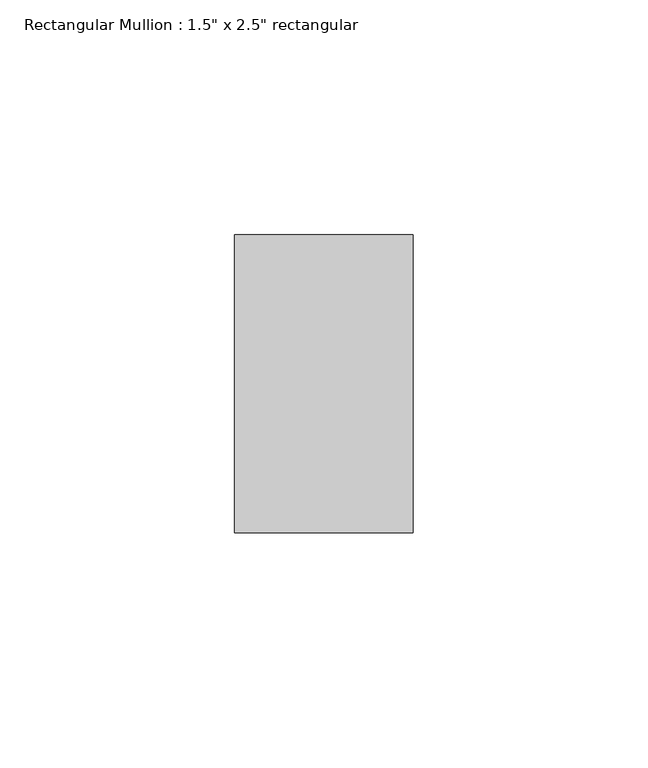
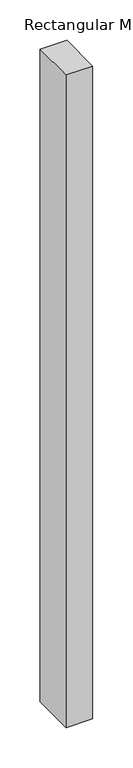
"""IFC4 building model written with IfcOpenShell, lengths in millimetres: member geometry."""

from ifc_helpers import new_model, si_unit, frame, origin, place, context, project, spatial, polyline, outline, extrude, source, transform, mapped, element, save


def member_e7145701(model_context):
    return source(origin(), model_context, "Body", "SweptSolid", [
        extrude(outline(polyline([(0.0, 31.75), (0.0, -31.75), (-38.1, -31.75), (-38.1, 31.75), (0.0, 31.75)])), frame((0.0, 0.0, -984.25), z_axis=(0.0, 0.0, 1.0), x_axis=(1.0, 0.0, 0.0)), (0.0, 0.0, 1.0), 984.25),
    ])


if __name__ == "__main__":
    model = new_model("IFC4")
    model_context = context("Model", 3, world=origin())
    ifc_project = project(units=[si_unit("LENGTHUNIT", "METRE", prefix="MILLI")], contexts=[model_context])
    site = spatial("IfcSite", under=ifc_project)
    building = spatial("IfcBuilding", under=site)
    placement = place(None, origin())
    member_shape = member_e7145701(model_context)
    element("IfcMember", 1, ObjectType="Rectangular Mullion : 1.5\" x 2.5\" rectangular", at=placement, inside=building, context=model_context, shape_type="MappedRepresentation", body=[
        mapped(member_shape, transform((0.0, 0.0, 0.0), x_axis=(1.0, 0.0, 0.0), y_axis=(0.0, 1.0, 0.0), z_axis=(0.0, 0.0, 1.0))),
    ])
    save(model, "model.ifc")

# Revit data of these elements
# Type "Rectangular Mullion : 1.5\" x 2.5\" rectangular"
#   built-in parameter 1007304 = 0.208333 (stored number, unit not read)
#   built-in parameter 1007301 = 0.0625 (stored number, unit not read)
#   built-in parameter 1007300 = 0.0625 (stored number, unit not read)
# Element 1 (IfcMember, "Rectangular Mullion : 1.5\" x 2.5\" rectangular")
#   Materials on its faces: "Aluminum"
# Materials
#   "Aluminum": class "Metal", colour RGB 247 247 247, transparency 0, Description = "Aluminum 6061", Cost = 0
